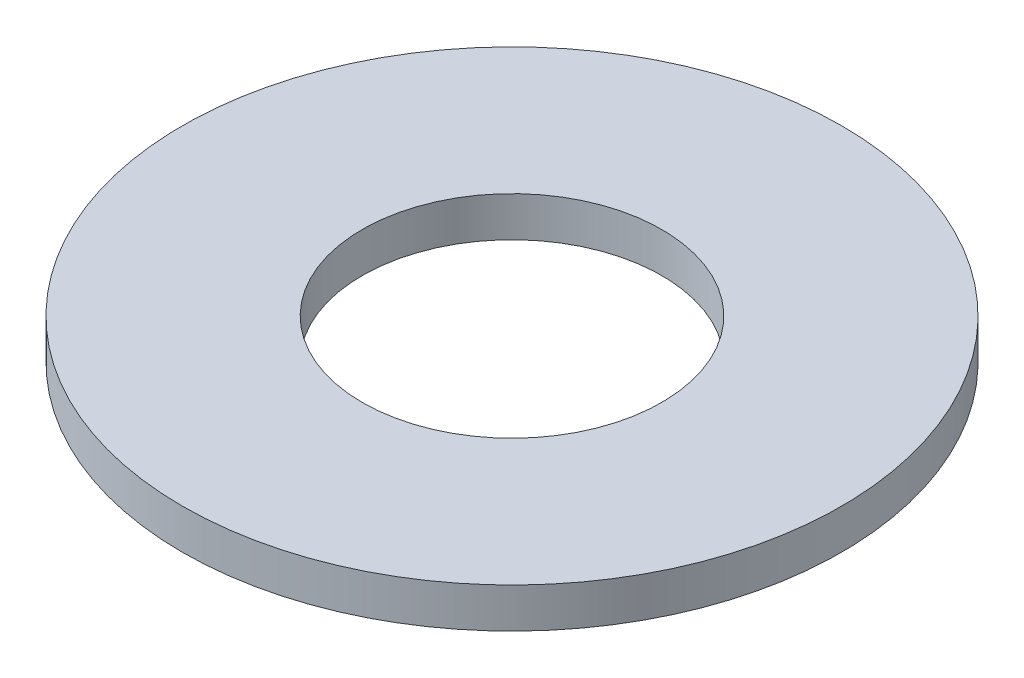
SolidWorks part; units mm, degrees
material "Plain Carbon Steel"
ref_plane "Front Plane" through (0, 0, 0) normal (0, 0, 1) x (1, 0, 0)
ref_plane "Top Plane" through (0, 0, 0) normal (0, 1, 0) x (1, 0, 0)
ref_plane "Right Plane" through (0, 0, 0) normal (1, 0, 0) x (0, 0, -1)
sketch "Washer Profile Ø165 x Ø75" plane through (0, 0, 0) normal (0, 1, 0) x (1, 0, 0)
  circle A0 centre (0, 0) radius 82.5
  circle A1 centre (0, 0) radius 37.5
  dimension "D1" = 75
  dimension "D2" = 165
extrude "Washer Body 10mm" add sketch "Washer Profile Ø165 x Ø75" along normal blind 10
